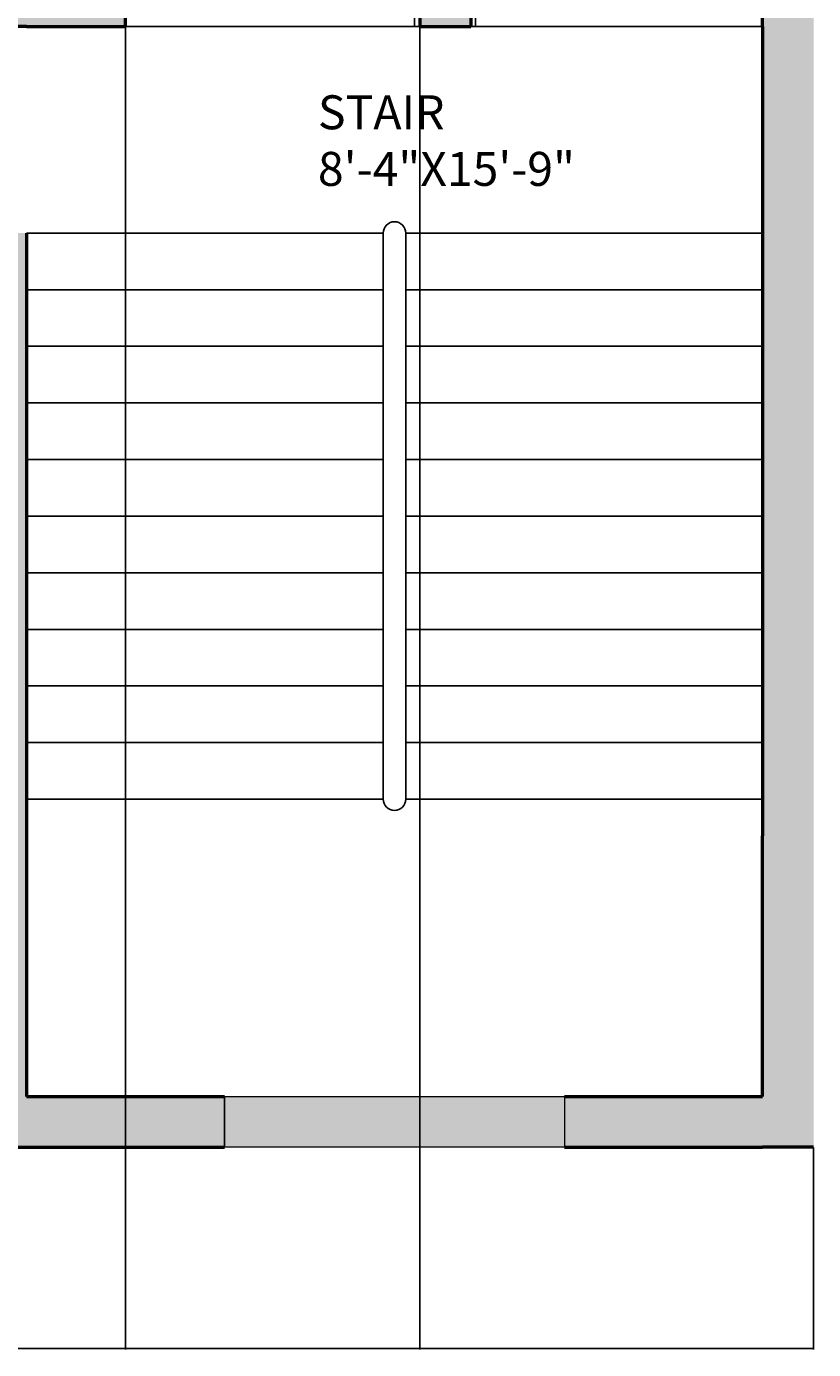
# Model space of a CAD drawing. Units: inches. Extents: x -12 to 604, y -566 to 58.
# Tile 2 of 12: x 249 to 388, y -566 to -332. Entities that reach past the tile are written whole.
import ezdxf

# ---------------------------------------------------------------- set-up
doc = ezdxf.new("R2010")
doc.units = ezdxf.units.IN
doc.header["$MEASUREMENT"] = 0
for name, color, linetype, lineweight in [('A-ANNO-DIMS', 2, 'Continuous', 18), ('A-AREA-IDEN', 7, 'Continuous', 18), ('A-DOOR', 4, 'Continuous', 25), ('A-FLOR-STRS', 7, 'Continuous', 25), ('A-GLAZ', 82, 'Continuous', 18), ('A-GLAZ-PATT', 82, 'Continuous', 13), ('A-WALL', 7, 'Continuous', 50), ('A-WALL-PATT', 18, 'Continuous', 13)]:
    doc.layers.add(name, color=color, linetype=linetype, lineweight=lineweight)
doc.styles.get("Standard").update_dxf_attribs({"font": 'arial.ttf'})
doc.dimstyles.get("Standard").update_dxf_attribs({"dimtxt": 0.18, "dimasz": 0.18, "dimexe": 0.18, "dimexo": 0.0625, "dimgap": 0.09, "dimtad": 0, "dimtih": 1, "dimtoh": 1, "dimdec": 0, "dimzin": 0, "dimdsep": 46, "dimlunit": 3, "dimtxsty": 'Standard', "dimcen": 0.09, "dimadec": 0, "dimazin": 0, "dimtfac": 1, "dimtdec": 0, "dimtofl": 0, "dimtmove": 0, "dimatfit": 3, "dimfxl": 1, "dimtolj": 1, "dimtzin": 0, "dimarcsym": 0})

# ---------------------------------------------------------------- blocks, each defined once
blk = doc.blocks.new('*D50')
at = {"layer": 'A-ANNO-DIMS', "color": 0, "lineweight": -2, "transparency": 16777216}
for p, q in [((240.32, -529.92), (240.32, -565.59)), ((388.32, -529.92), (388.32, -565.59)), ((240.5, -565.41), (313.93, -565.41)), ((388.14, -565.41), (314.71, -565.41))]:
    blk.add_line(p, q, dxfattribs=at)
at = {"layer": 'A-ANNO-DIMS', "color": 0, "transparency": 16777216}
for points in [[(240.5, -565.38), (240.5, -565.44), (240.32, -565.41)], [(388.14, -565.38), (388.14, -565.44), (388.32, -565.41)]]:
    blk.add_solid(points, dxfattribs=at)
at = {"layer": 'Defpoints', "color": 0, "transparency": 16777216}
for p in [(240.32, -529.86), (388.32, -529.86), (388.32, -565.41)]:
    blk.add_point(p, dxfattribs=at)
at = {"layer": 'A-ANNO-DIMS', "color": 0, "transparency": 16777216, "insert": (314.32, -565.41), "char_height": 0.18, "attachment_point": 5}
blk.add_mtext('\\A1;12\'-4"', dxfattribs=at)
blk = doc.blocks.new('*D55')
at = {"layer": 'A-ANNO-DIMS', "color": 0, "lineweight": -2, "transparency": 16777216}
for p, q in [((266.82, -331.92), (266.82, -565.59)), ((318.82, -331.92), (318.82, -565.59)), ((267, -565.41), (292.49, -565.41)), ((318.64, -565.41), (293.16, -565.41))]:
    blk.add_line(p, q, dxfattribs=at)
at = {"layer": 'A-ANNO-DIMS', "color": 0, "transparency": 16777216}
for points in [[(267, -565.38), (267, -565.44), (266.82, -565.41)], [(318.64, -565.38), (318.64, -565.44), (318.82, -565.41)]]:
    blk.add_solid(points, dxfattribs=at)
at = {"layer": 'Defpoints', "color": 0, "transparency": 16777216}
for p in [(266.82, -331.86), (318.82, -331.86), (318.82, -565.41)]:
    blk.add_point(p, dxfattribs=at)
at = {"layer": 'A-ANNO-DIMS', "color": 0, "transparency": 16777216, "insert": (292.82, -565.41), "char_height": 0.18, "attachment_point": 5}
blk.add_mtext('\\A1;4\'-4"', dxfattribs=at)

msp = doc.modelspace()

# ---------------------------------------------------------------- hatches: boundary and pattern name
at = {"layer": 'A-GLAZ-PATT'}
h = msp.add_hatch(dxfattribs=at)
h.set_pattern_fill('GOST_WOOD', color=256)
h.set_pattern_definition([(90, (0, 0), (6, -4e-16), [10, -2]), (90, (2, -2), (6, -4e-16), [6, -1.5, 3, -1.5]), (90, (4, -5), (6, -4e-16), [10, -2])])
h.paths.add_polyline_path([(344.32, -529.86), (344.32, -520.86), (284.32, -520.86), (284.32, -529.86)])
h.paths.add_polyline_path([(604.32, -450.86), (598.32, -450.86), (598.32, -474.86), (604.32, -474.86)])
h.paths.add_polyline_path([(598.32, -309.28), (604.32, -309.28), (604.32, -274.86), (598.32, -274.86)])
h.paths.add_polyline_path([(598.32, -235.86), (604.32, -235.86), (604.32, -204.86), (598.32, -204.86)])
h.paths.add_polyline_path([(598.32, -159.86), (604.32, -159.86), (604.32, -99.86), (598.32, -99.86)])
at = {"layer": 'A-WALL-PATT'}
h = msp.add_hatch(color=256, dxfattribs=at)
h.dxf.hatch_style = 1
h.paths.add_polyline_path([(169.32, 11.14), (169.32, 17.14), (160.32, 17.14), (160.32, 11.14), (118.32, 11.14), (118.32, 6.64), (118.32, 2.14), (127.32, 2.14), (169.32, 2.14)])
h.paths.add_polyline_path([(127.32, -13.61), (118.32, -13.61), (118.32, -29.36), (34.82, -29.36), (24.32, -29.36), (24.32, -38.36), (39.32, -38.36), (118.32, -38.36), (118.32, -126.86), (127.32, -126.86), (127.32, -117.86)])
h.paths.add_polyline_path([(82.32, -92.36), (39.32, -92.36), (39.32, -56.22), (30.32, -56.22), (24.32, -56.22), (24.32, -65.22), (30.32, -65.22), (30.32, -113.36), (24.32, -113.36), (24.32, -122.36), (39.32, -122.36), (39.32, -101.36), (82.32, -101.36), (82.32, -96.86)], flags=17)
h.paths.add_polyline_path([(280.32, 11.14), (238.32, 11.14), (238.32, 17.14), (229.32, 17.14), (229.32, 12.64), (229.32, 11.14), (229.32, 2.14), (271.32, 2.14), (271.32, -117.86), (163.32, -117.86), (163.32, -126.86), (271.32, -126.86), (271.32, -189.86), (280.32, -189.86), (280.32, -180.86)])
h.paths.add_polyline_path([(415.32, 17.14), (406.32, 17.14), (406.32, 11.14), (358.32, 11.14), (358.32, -21.86), (367.32, -21.86), (367.32, 2.14), (415.32, 2.14)], flags=17)
h.paths.add_polyline_path([(484.55, -45.86), (448.32, -45.86), (448.32, 2.14), (448.32, 17.14), (439.32, 17.14), (439.32, 12.64), (439.32, 2.14), (439.32, -45.86), (367.32, -45.86), (358.32, -45.86), (358.32, -54.86), (430.32, -54.86), (430.32, -69.59), (430.32, -180.86), (318.82, -180.86), (318.82, -189.86), (318.82, -331.86), (327.82, -331.86), (327.82, -189.86), (439.32, -189.86), (439.32, -180.86), (439.32, -54.86), (483.5, -54.86), (484.55, -54.86)])
h.paths.add_polyline_path([(529.32, 11.14), (481.32, 11.14), (481.32, 17.14), (472.32, 17.14), (472.32, 12.64), (472.32, 2.14), (520.32, 2.14), (520.32, -21.86), (529.32, -21.86)])
h.paths.add_polyline_path([(598.32, -45.86), (582.42, -45.86), (582.42, -50.36), (582.42, -54.86), (589.32, -54.86), (589.32, -99.86), (598.32, -99.86), (604.32, -99.86), (604.32, -90.86), (598.32, -90.86)])
h.paths.add_polyline_path([(598.32, -168.86), (604.32, -168.86), (604.32, -159.86), (589.32, -159.86), (589.32, -180.86), (477.32, -180.86), (477.32, -189.86), (477.32, -259.86), (486.32, -259.86), (486.32, -189.86), (589.32, -189.86), (589.32, -204.86), (598.32, -204.86), (604.32, -204.86), (604.32, -195.86), (598.32, -195.86)])
h.paths.add_polyline_path([(598.32, -244.86), (604.32, -244.86), (604.32, -235.86), (598.32, -235.86), (589.32, -235.86), (589.32, -250.86), (522.32, -250.86), (522.32, -259.86), (589.32, -259.86), (589.32, -274.86), (598.32, -274.86), (604.32, -274.86), (604.32, -265.86), (598.32, -265.86)])
h.paths.add_polyline_path([(598.32, -333.28), (604.32, -333.28), (604.32, -324.28), (598.32, -324.28), (598.32, -321.87), (598.32, -318.28), (604.32, -318.28), (604.32, -309.28), (598.32, -309.28), (589.32, -309.28), (589.32, -341.95), (589.38, -341.95), (589.38, -363.16), (589.32, -381.86), (565.32, -381.86), (565.32, -390.86), (589.32, -390.86), (589.32, -450.86), (598.32, -450.86), (604.32, -450.86), (604.32, -441.86), (598.32, -441.86), (598.32, -390.86), (604.32, -390.86), (604.32, -381.86), (598.32, -381.86)])
h.paths.add_polyline_path([(541.32, -345.86), (424.32, -345.86), (424.32, -354.86), (532.32, -354.86), (532.32, -474.86), (463.39, -474.86), (463.39, -483.86), (553.32, -483.86), (553.32, -474.86), (541.32, -474.86), (541.32, -390.86), (541.32, -381.86)])
h.paths.add_polyline_path([(604.32, -474.86), (589.32, -474.86), (553.32, -474.86), (553.32, -483.86), (598.32, -483.86), (604.32, -483.86)])
h.paths.add_polyline_path([(388.32, -483.86), (388.32, -474.86), (388.32, -460.13), (388.32, -333.86), (388.32, -322.86), (379.32, -322.86), (379.32, -331.86), (379.32, -333.86), (379.32, -474.86), (379.32, -520.86), (344.32, -520.86), (344.32, -529.86), (379.32, -529.86), (388.32, -529.86)])
h.paths.add_polyline_path([(284.32, -520.86), (249.32, -520.86), (249.32, -474.86), (249.32, -368.36), (240.32, -368.36), (240.32, -474.86), (238.52, -474.86), (238.52, -483.86), (240.32, -483.86), (240.32, -529.86), (249.32, -529.86), (284.32, -529.86)])
h.paths.add_polyline_path([(178.82, -474.86), (158.91, -474.86), (158.91, -483.86), (162.32, -483.86), (178.82, -483.86)])
h.paths.add_polyline_path([(84.32, -474.86), (84.32, -366.86), (75.32, -366.86), (75.32, -474.86), (39.32, -474.86), (39.32, -453.86), (24.32, -453.86), (24.32, -462.86), (30.32, -462.86), (30.32, -483.86), (84.32, -483.86)])
h.paths.add_polyline_path([(39.32, -342.86), (75.32, -342.86), (84.32, -342.86), (179.67, -342.86), (179.67, -333.86), (39.32, -333.86), (39.32, -318.86), (24.32, -318.86), (24.32, -327.86), (30.32, -327.86), (30.32, -432.86), (24.32, -432.86), (24.32, -441.86), (30.32, -441.86), (39.32, -441.86)])
h.paths.add_polyline_path([(249.32, -252.86), (115.32, -252.86), (115.32, -225.86), (106.32, -225.86), (106.32, -252.86), (39.32, -252.86), (39.32, -237.86), (24.32, -237.86), (24.32, -246.86), (30.32, -246.86), (30.32, -267.86), (24.32, -267.86), (24.32, -276.86), (39.32, -276.86), (39.32, -261.86), (240.32, -261.86), (240.32, -331.86), (249.32, -331.86), (266.82, -331.86), (266.82, -322.86), (249.32, -322.86)])
h.paths.add_polyline_path([(127.32, -180.86), (39.32, -180.86), (24.32, -180.86), (24.32, -189.86), (39.32, -189.86), (127.32, -189.86)])
h.paths.add_polyline_path([(39.32, -159.86), (24.32, -159.86), (24.32, -168.86), (30.32, -168.86), (30.32, -180.86), (39.32, -180.86)])
h.paths.add_polyline_path([(470.51, -17.27), (512.48, -17.27), (512.48, 5.12), (470.51, 5.12)], flags=9)
h.paths.add_polyline_path([(484.21, -244.26), (526.45, -244.26), (526.45, -221.87), (484.21, -221.87)], flags=24)
h.paths.add_polyline_path([(36.91, -442.88), (83.54, -442.88), (83.54, -420.5), (36.91, -420.5)], flags=25)

# ---------------------------------------------------------------- linework, layer by layer
at = {"layer": 'A-DOOR'}
for p, q in [((317.86, -331.86), (317.86, -295.86)), ((328.6, -331.86), (328.6, -295.86)), ((318.82, -331.86), (266.82, -331.86)), ((327.82, -331.86), (379.32, -331.86))]:
    msp.add_line(p, q, dxfattribs=at)
at = {"layer": 'A-FLOR-STRS'}
for p, q in [((312.32, -368.36), (249.32, -368.36)), ((312.32, -368.36), (312.32, -468.36)), ((316.32, -368.36), (316.32, -468.36)), ((316.32, -368.36), (379.32, -368.36)), ((312.32, -378.36), (249.32, -378.36)), ((316.32, -378.36), (379.32, -378.36)), ((312.32, -388.36), (249.32, -388.36)), ((316.32, -388.36), (379.32, -388.36)), ((312.32, -398.36), (249.32, -398.36)), ((316.32, -398.36), (379.32, -398.36)), ((312.32, -408.36), (249.32, -408.36)), ((316.32, -408.36), (379.32, -408.36)), ((312.32, -418.36), (249.32, -418.36)), ((316.32, -418.36), (379.32, -418.36)), ((312.32, -428.36), (249.32, -428.36)), ((316.32, -428.36), (379.32, -428.36)), ((312.32, -438.36), (249.32, -438.36)), ((312.32, -438.36), (249.32, -438.36)), ((316.32, -438.36), (379.32, -438.36)), ((312.32, -448.36), (249.32, -448.36)), ((316.32, -448.36), (379.32, -448.36)), ((312.32, -458.36), (249.32, -458.36)), ((316.32, -458.36), (379.32, -458.36)), ((312.32, -468.36), (249.32, -468.36)), ((316.32, -468.36), (379.32, -468.36))]:
    msp.add_line(p, q, dxfattribs=at)
for centre, start, end in [((314.32, -368.36), 0, 180), ((314.32, -468.36), 180, 0)]:
    msp.add_arc(centre, 2, start, end, dxfattribs=at)
at = {"layer": 'A-GLAZ'}
for p, q in [((284.32, -520.86), (284.32, -529.86)), ((284.32, -520.86), (344.32, -520.86)), ((284.32, -529.86), (284.32, -520.86)), ((344.32, -520.86), (344.32, -529.86)), ((344.32, -520.86), (344.32, -529.86)), ((344.32, -529.86), (284.32, -529.86))]:
    msp.add_line(p, q, dxfattribs=at)
at = {"layer": 'A-WALL'}
for p, q in [((318.82, -180.86), (318.82, -331.86)), ((327.82, -189.86), (327.82, -331.86)), ((266.82, -331.86), (266.82, -322.86)), ((379.32, -331.86), (379.32, -322.86)), ((249.32, -331.86), (240.32, -331.86)), ((249.32, -331.86), (266.82, -331.86)), ((318.82, -331.86), (327.82, -331.86)), ((379.32, -331.86), (379.32, -333.86)), ((379.32, -333.86), (379.32, -474.86)), ((249.32, -368.36), (249.32, -474.86)), ((249.32, -474.86), (249.32, -520.86)), ((379.32, -520.86), (379.32, -474.86)), ((249.32, -520.86), (284.32, -520.86)), ((344.32, -520.86), (379.32, -520.86)), ((240.32, -529.86), (249.32, -529.86)), ((249.32, -529.86), (284.32, -529.86)), ((344.32, -529.86), (379.32, -529.86)), ((388.32, -529.86), (379.32, -529.86))]:
    msp.add_line(p, q, dxfattribs=at)

# ---------------------------------------------------------------- texts
at = {"layer": 'A-AREA-IDEN', "insert": (300.8, -344.02), "char_height": 6, "attachment_point": 1}
msp.add_mtext('STAIR\\P8\'-4"X15\'-9"', dxfattribs=at)

# ---------------------------------------------------------------- dimensions: what is measured, and where the dimension line sits
at = {"layer": 'A-ANNO-DIMS'}
for base, p1, p2, picture, middle in [((318.82, -565.41), (266.82, -331.86), (318.82, -331.86), '*D55', (292.82, -565.41)), ((388.32, -565.41), (240.32, -529.86), (388.32, -529.86), '*D50', (314.32, -565.41))]:
    dim = msp.add_linear_dim(base=base, p1=p1, p2=p2, dimstyle='Standard', override={"dimdec": 1, "dimlfac": 1, "dimrnd": 0, "dimzin": 1, "dimdsep": 46, "dimlunit": 4, "dimfrac": 2}, dxfattribs=at)
    dim.commit()
    dim.dimension.update_dxf_attribs({"geometry": picture, "text_midpoint": middle})

doc.saveas('drawing.dxf')
